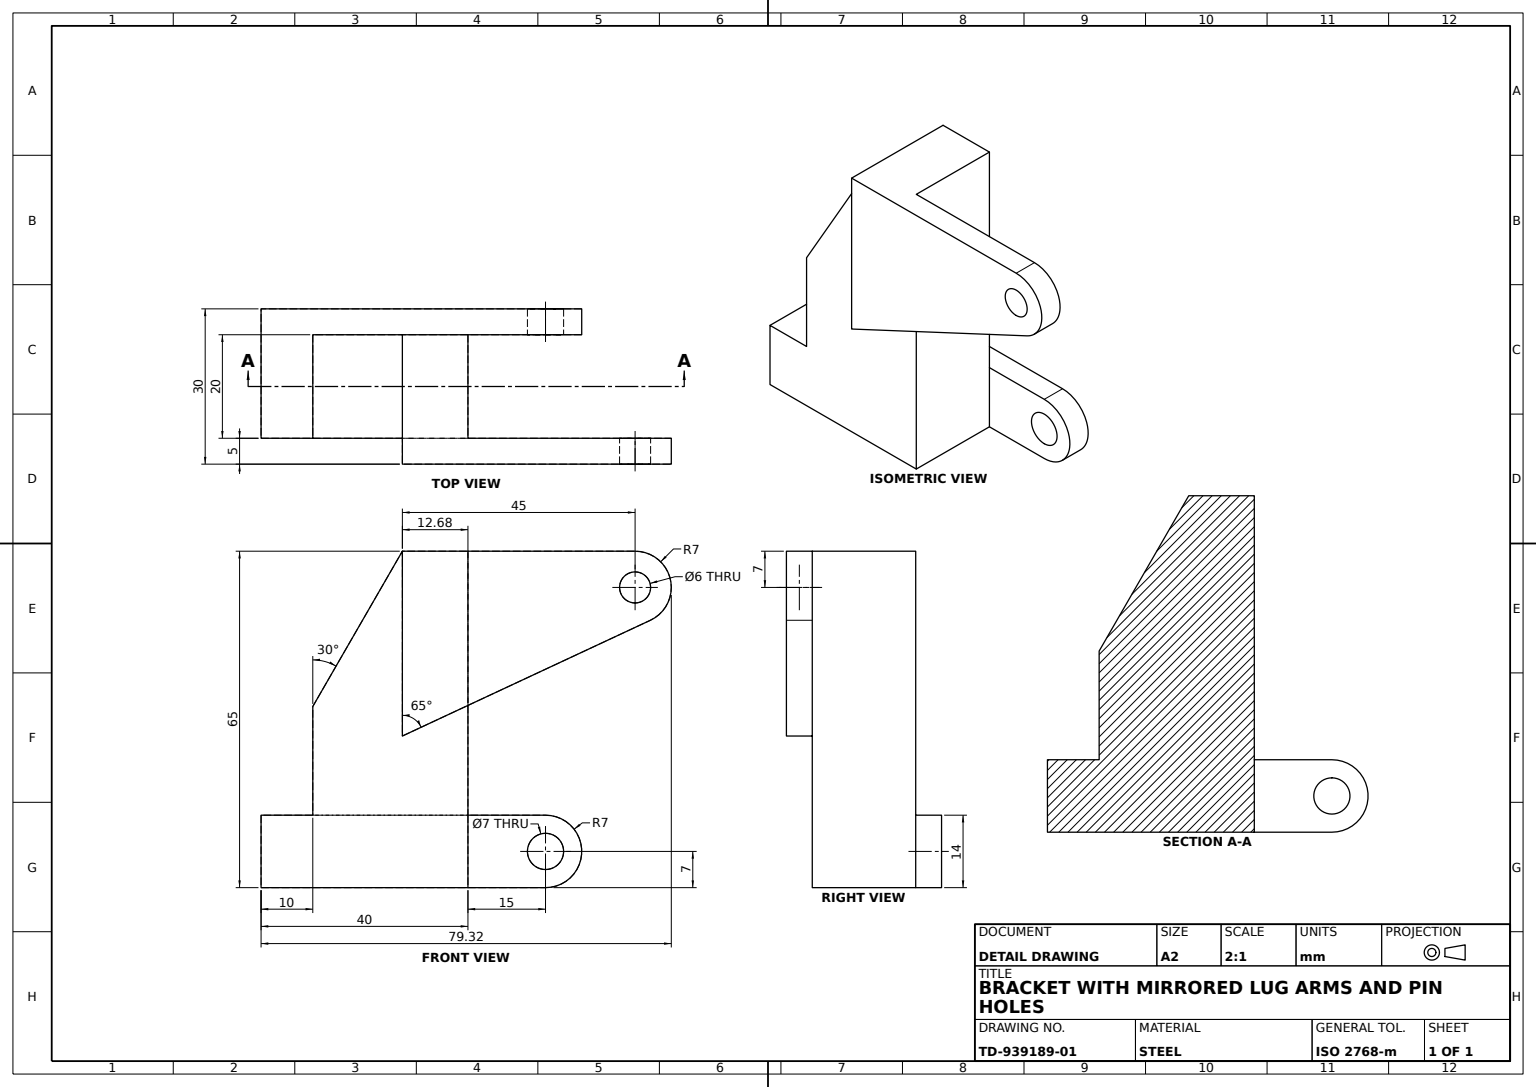
SolidWorks part; units mm, degrees
material "Plain Carbon Steel"
ref_plane "Front Plane" through (0, 0, 0) normal (0, 0, 1) x (1, 0, 0)
ref_plane "Top Plane" through (0, 0, 0) normal (0, 1, 0) x (1, 0, 0)
ref_plane "Right Plane" through (0, 0, 0) normal (1, 0, 0) x (0, 0, -1)
sketch "Base Block Sketch" plane through (0, 0, 0) normal (0, 0, 1) x (1, 0, 0)
  line L1 (-10, 32.5) -> (10, 32.5)
  line L2 (-10, 32.5) -> (-10, -32.5)
  line L3 (-10, -32.5) -> (10, -32.5)
  line L4 (10, 32.5) -> (10, -32.5)
  line L5 (-10, 32.5) -> (10, -32.5) construction
  line L6 (-10, -32.5) -> (10, 32.5) construction
  point P0 (0, 0)
  dimension "D1" = 20
  dimension "D2" = 65
extrude "Base Block" add sketch "Base Block Sketch" along normal blind 40
sketch "Angled Cut Sketch" plane through (10, 0, 0) normal (1, 0, 0) x (0, 0, -1)
  line L0 (-12.6795, 32.5) -> (-30, 2.5)
  line L1 (0, 0) -> (-74.1746, 0) construction
  line L2 (-40, -32.5) -> (-40, 32.5) construction
  line L3 (-30, -18.5) -> (-30, 2.5)
  line L4 (-30, -18.5) -> (-40, -18.5)
  line L9 (-40, 32.5) -> (-12.6795, 32.5)
  line L10 (-40, 32.5) -> (-40, -18.5)
  line L13 (-40, -32.5) -> (0, -32.5) construction
  line L14 (0, -32.5) -> (0, 32.5) construction
  dimension "D1" = 30
  dimension "D2" = 14
  dimension "D3" = 12.6795
  dimension "D4" = 30
extrude "Angled Cut 30deg" cut sketch "Angled Cut Sketch" against normal through all both and the other way through all
sketch "Side Pad Sketch" plane through (10, 0, 0) normal (1, 0, 0) x (0, 0, -1)
  line L0 (0, -32.5) -> (0, 32.5) construction
  line L1 (-40, -32.5) -> (15, -32.5)
  line L2 (-40, -32.5) -> (-40, -18.5)
  line L3 (-40, -18.5) -> (15, -18.5)
  arc A0 (15, -32.5) -> (15, -18.5) centre (15, -25.5) ccw
  dimension "D1" = 14
  dimension "D2" = 15
extrude "Side Pad" add sketch "Side Pad Sketch" along normal blind 5
mirror "Side Pad Mirror" about plane through (0, 0, 0) normal (1, 0, 0) of "Side Pad"
sketch "Pad Trim Sketch" plane through (15, 0, 0) normal (1, 0, 0) x (0, 0, -1)
  line L3 (-40, -18.5) -> (-40, -32.5)
  line L4 (-40, -32.5) -> (15, -32.5)
  line L5 (15, -18.5) -> (-40, -18.5)
  line L6 (-40, -18.5) -> (-40, -32.5)
  line L7 (-40, -32.5) -> (15, -32.5)
  line L8 (15, -18.5) -> (-40, -18.5)
  arc A1 (15, -32.5) -> (15, -18.5) centre (15, -25.5) ccw
  arc A2 (15, -32.5) -> (15, -18.5) centre (15, -25.5) ccw
  dimension "D1" = 0
extrude "Pad Trim Cut" cut sketch "Pad Trim Sketch" against normal blind 5 and the other way through all
sketch "Pin Hole Sketch" plane through (-10, 0, 0) normal (1, 0, 0) x (0, 0, -1)
  circle A0 centre (15, -25.5) radius 3.5
  dimension "D1" = 7
extrude "Pin Hole Ø7" cut sketch "Pin Hole Sketch" against normal blind 5
sketch "Lever Arm Sketch" plane through (10, 0, 0) normal (1, 0, 0) x (0, 0, -1)
  line L0 (-12.6795, 32.5) -> (-12.6795, -3.2075)
  line L1 (-12.6795, -3.2075) -> (35.2788, 19.1558)
  line L2 (-12.6795, 32.5) -> (32.3205, 32.5)
  arc A0 (35.2788, 19.1558) -> (32.3205, 32.5) centre (32.3205, 25.5) ccw
  circle A1 centre (32.3205, 25.5) radius 3
  dimension "D2" = 14
  dimension "D4" = 6
  dimension "D1" = 65
  dimension "D3" = 45
extrude "Lever Arm" add sketch "Lever Arm Sketch" along normal blind 5
